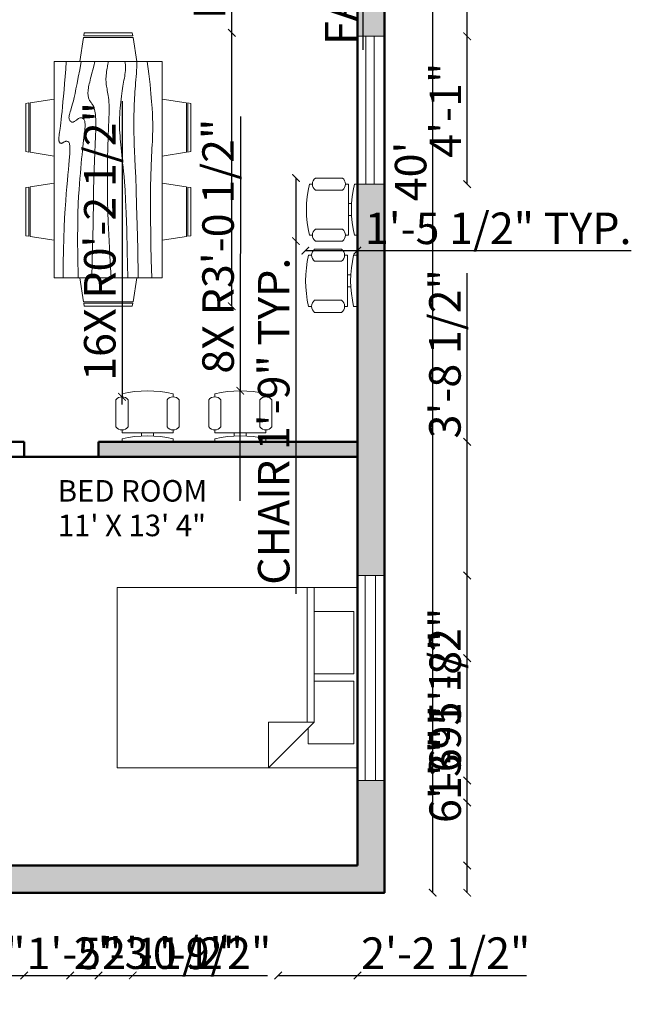
# Model space of a CAD drawing. Units: inches. Extents: x 1699 to 2290, y 1404 to 1978.
# Tile 3 of 4: x 2086 to 2290, y 1404 to 1732. Entities that reach past the tile are written whole.
import ezdxf

# ---------------------------------------------------------------- set-up
doc = ezdxf.new("R2010")
doc.units = ezdxf.units.IN
for name, color, linetype, lineweight in [('A-ANNO-DIMS', 2, 'Continuous', 18), ('A-AREA-IDEN', 7, 'Continuous', 25), ('A-FURN', 8, 'Continuous', 18), ('A-WALL', 7, 'Continuous', 50), ('A-WALL-PATT', 17, 'Continuous', 13), ('window', 3, 'Continuous', 18)]:
    doc.layers.add(name, color=color, linetype=linetype, lineweight=lineweight)
doc.styles.get("Standard").update_dxf_attribs({"font": 'arial.ttf'})
doc.dimstyles.new('ISO-25', dxfattribs={"dimtxt": 10.5, "dimasz": 2.5, "dimexe": 1.25, "dimexo": 0.625, "dimtad": 1, "dimdec": 0, "dimlunit": 4, "dimtxsty": 'Standard', "dimblk": 'ARCHTICK', "dimcen": 2.5, "dimse1": 1, "dimse2": 1, "dimclrd": 4, "dimclrt": 2, "dimadec": 0, "dimazin": 0, "dimtfac": 1, "dimtdec": 0, "dimtmove": 0, "dimatfit": 3, "dimfxl": 1, "dimarcsym": 0})

# ---------------------------------------------------------------- blocks, each defined once
blk = doc.blocks.new('Bed - Queen')
for p, q in [((0, -80.00003), (0, 0)), ((0, 0), (59.99999, 0)), ((59.99999, 0), (59.99999, -80.00003)), ((7.99999, -1.2), (28.79998, -1.2)), ((7.99999, -14.4), (7.99999, -1.2)), ((28.79998, -1.2), (28.79998, -14.4)), ((31.19999, -1.2), (51.99999, -1.2)), ((31.19999, -14.4), (31.19999, -1.2)), ((51.99999, -1.2), (51.99999, -16.4)), ((0, -14.4), (44.8, -14.4)), ((59.99999, -29.6), (44.8, -14.4)), ((44.8, -14.4), (44.8, -29.6)), ((44.8, -16.8), (0, -16.8)), ((51.99999, -16.4), (46.79936, -16.4)), ((44.8, -29.6), (59.99999, -29.6)), ((59.99999, -80.00003), (0, -80.00003))]:
    blk.add_line(p, q)
blk = doc.blocks.new('Dining Set - 36 x 72 in.')
for p, q in [((-22, 27.5), (-22.1562, 26.50042)), ((-5.8416, 26.5), (-22.1534, 26.5)), ((-22, 27.5), (-6, 27.5)), ((-5.8437, 26.49966), (-6, 27.5)), ((6, 27.5), (5.8438, 26.50042)), ((22.1584, 26.5), (5.8466, 26.5)), ((6, 27.5), (22, 27.5)), ((22.1563, 26.49966), (22, 27.5)), ((-22.2343, 26.00059), (-23.4847, 17.99762)), ((-22.2304, 26), (-5.7608, 26)), ((-4.5152, 17.99762), (-5.7655, 25.99926)), ((5.7657, 26.00059), (4.5153, 17.99762)), ((5.7696, 26), (22.2392, 26)), ((23.4848, 17.99762), (22.2345, 25.99926)), ((36, 18), (-36, 18)), ((-36, 18), (-36, -18)), ((36, -18), (36, 18)), ((-45.5, 8), (-44.5004, 8.15617)), ((-45.5, 8), (-45.5, -8)), ((-44.5, -8.15843), (-44.5, 8.15338)), ((-44.0006, 8.23428), (-35.9976, 9.48474)), ((-44, 8.23041), (-44, -8.23915)), ((44.0006, 8.23428), (35.9976, 9.48474)), ((44, 8.23041), (44, -8.23915)), ((44.5, -8.15843), (44.5, 8.15338)), ((45.5, 8), (44.5005, 8.15617)), ((45.5, 8), (45.5, -8)), ((-44.4997, -8.15631), (-45.5, -8)), ((-35.9976, -9.48476), (-43.9993, -8.2345)), ((35.9976, -9.48476), (43.9993, -8.2345)), ((44.4997, -8.15631), (45.5, -8)), ((-36, -18), (36, -18)), ((-22.2343, -26.0006), (-23.4847, -17.99762)), ((-4.5152, -17.99762), (-5.7655, -25.99928)), ((5.7657, -26.0006), (4.5153, -17.99762)), ((23.4848, -17.99762), (22.2345, -25.99928)), ((-22.2304, -26), (-5.7608, -26)), ((5.7696, -26), (22.2392, -26)), ((-22, -27.5), (-22.1562, -26.50044)), ((-5.8416, -26.5), (-22.1534, -26.5)), ((-22, -27.5), (-6, -27.5)), ((-5.8437, -26.49967), (-6, -27.5)), ((6, -27.5), (5.8438, -26.50044)), ((22.1584, -26.5), (5.8466, -26.5)), ((6, -27.5), (22, -27.5)), ((22.1563, -26.49967), (22, -27.5))]:
    blk.add_line(p, q)
for points in [[(-36, 15), (-31.1772, 14.97754), (-26.8079, 14.91406), (-22.8538, 14.81543), (-19.276, 14.6875), (-16.0362, 14.53613), (-13.0957, 14.36718), (-10.4159, 14.18652), (-7.9583, 14), (-5.6904, 13.81315), (-3.6035, 13.63021), (-1.6954, 13.45508), (0.0365, 13.29166), (1.5945, 13.14388), (2.9811, 13.01562), (4.1988, 12.9108), (5.25, 12.83333), (6.1393, 12.78613), (6.8802, 12.76823), (7.4883, 12.77767), (7.9792, 12.8125), (8.3685, 12.87077), (8.6719, 12.95052), (8.9049, 13.0498), (9.0833, 13.16666), (9.2205, 13.29899), (9.3216, 13.44401), (9.3895, 13.59879), (9.4271, 13.76041), (9.4373, 13.92594), (9.4232, 14.09245), (9.3875, 14.257), (9.3333, 14.41666), (9.2638, 14.56917), (9.1836, 14.71484), (9.0975, 14.85465), (9.0104, 14.98958), (8.9272, 15.1206), (8.8529, 15.2487), (8.7922, 15.37483), (8.75, 15.5), (8.7305, 15.62467), (8.7344, 15.74739), (8.7617, 15.86621), (8.8125, 15.97916), (8.8867, 16.08431), (8.9844, 16.17968), (9.1055, 16.26334), (9.25, 16.33333), (9.4189, 16.38802), (9.6172, 16.42708), (9.8506, 16.45052), (10.125, 16.45833), (10.4463, 16.45052), (10.8203, 16.42708), (11.2529, 16.38802), (11.75, 16.33333), (12.3184, 16.26318), (12.9694, 16.17838), (13.7151, 16.07991), (14.5677, 15.96875), (15.5395, 15.84586), (16.6426, 15.71224), (17.8893, 15.56884), (19.2917, 15.41666), (20.859, 15.25667), (22.5879, 15.08984), (24.4721, 14.91715), (26.5052, 14.73958), (28.6809, 14.5581), (30.9929, 14.3737), (33.4347, 14.18733), (36, 14)], [(-36, 10), (-28.9766, 10.14274), (-23.1725, 10.20442), (-18.4241, 10.19775), (-14.5677, 10.13541), (-11.4399, 10.03011), (-8.877, 9.89453), (-6.7154, 9.74137), (-4.7917, 9.58333), (-2.9698, 9.43082), (-1.2246, 9.28515), (0.4415, 9.14534), (2.026, 9.01041), (3.5266, 8.87939), (4.9408, 8.7513), (6.266, 8.62516), (7.5, 8.5), (8.6411, 8.37549), (9.6914, 8.2539), (10.6538, 8.13818), (11.5312, 8.03125), (12.3267, 7.93603), (13.043, 7.85547), (13.6831, 7.79248), (14.25, 7.75), (14.7471, 7.7303), (15.1797, 7.73307), (15.5537, 7.75732), (15.875, 7.80208), (16.1494, 7.86637), (16.3828, 7.94922), (16.5811, 8.04964), (16.75, 8.16666), (16.8944, 8.29915), (17.0143, 8.44531), (17.1089, 8.60319), (17.1771, 8.77083), (17.218, 8.94629), (17.2305, 9.1276), (17.2137, 9.31282), (17.1667, 9.5), (17.0895, 9.6875), (16.987, 9.875), (16.8649, 10.0625), (16.7292, 10.25), (16.5856, 10.4375), (16.4401, 10.625), (16.2985, 10.8125), (16.1667, 11), (16.05, 11.18733), (15.9518, 11.3737), (15.8752, 11.5581), (15.8229, 11.73958), (15.798, 11.91715), (15.8034, 12.08984), (15.842, 12.25667), (15.9167, 12.41666), (16.0295, 12.56836), (16.1784, 12.70833), (16.3605, 12.83268), (16.5729, 12.9375), (16.8127, 13.01888), (17.0768, 13.07291), (17.3625, 13.0957), (17.6667, 13.08333), (17.9894, 13.03312), (18.3418, 12.94726), (18.7382, 12.82918), (19.1927, 12.68229), (19.7195, 12.51001), (20.3327, 12.31575), (21.0465, 12.10294), (21.875, 11.875), (22.8357, 11.63354), (23.959, 11.37304), (25.2786, 11.08618), (26.8282, 10.76562), (28.6414, 10.40405), (30.752, 9.99414), (33.1936, 9.52856), (36, 9)], [(-36, 5.5), (-30.7157, 5.3348), (-26.069, 5.20963), (-21.9946, 5.11767), (-18.4271, 5.05208), (-15.3009, 5.00602), (-12.5508, 4.97265), (-10.1112, 4.94515), (-7.9167, 4.91666), (-5.909, 4.88167), (-4.0586, 4.83984), (-2.3429, 4.79215), (-0.7396, 4.73958), (0.7739, 4.6831), (2.22, 4.6237), (3.6213, 4.56233), (5, 4.5), (6.373, 4.43782), (7.7344, 4.3776), (9.0723, 4.32129), (10.375, 4.27083), (11.6309, 4.22819), (12.8281, 4.19531), (13.9551, 4.17415), (15, 4.16666), (15.954, 4.17448), (16.819, 4.19791), (17.6001, 4.23698), (18.3021, 4.29166), (18.9299, 4.36198), (19.4883, 4.44791), (19.9823, 4.54948), (20.4167, 4.66666), (20.7969, 4.79899), (21.1302, 4.94401), (21.4245, 5.09879), (21.6875, 5.26041), (21.9271, 5.42594), (22.1511, 5.59245), (22.3672, 5.757), (22.5834, 5.91666), (22.8065, 6.06868), (23.0404, 6.21093), (23.2879, 6.34147), (23.5521, 6.45833), (23.8358, 6.55957), (24.142, 6.64323), (24.4735, 6.70735), (24.8334, 6.75), (25.2235, 6.76969), (25.642, 6.76692), (26.0858, 6.74267), (26.5521, 6.69791), (27.0379, 6.63362), (27.5404, 6.55078), (28.0565, 6.45036), (28.5834, 6.33333), (29.1242, 6.19987), (29.7071, 6.04687), (30.3661, 5.87044), (31.1354, 5.66666), (32.0493, 5.43164), (33.142, 5.16146), (34.4475, 4.85221), (36, 4.5)], [(-36, -1), (-30.7915, -0.6591), (-26.0195, -0.38216), (-21.6519, -0.16284), (-17.6563, 0.00521), (-14.0005, 0.12833), (-10.6523, 0.21289), (-7.5796, 0.26522), (-4.75, 0.29166), (-2.134, 0.29793), (0.2878, 0.28711), (2.5317, 0.26163), (4.6146, 0.22396), (6.5529, 0.17651), (8.3633, 0.12174), (10.0623, 0.06209), (11.6667, 0), (13.1899, -0.06201), (14.6341, -0.1211), (15.9982, -0.17432), (17.2813, -0.21875), (18.4823, -0.25147), (19.6003, -0.26953), (20.6343, -0.27002), (21.5834, -0.25), (22.4481, -0.20768), (23.2357, -0.14584), (23.9549, -0.06836), (24.6146, 0.02083), (25.2235, 0.11784), (25.7904, 0.21875), (26.3241, 0.31966), (26.8334, 0.41666), (27.3265, 0.50618), (27.8099, 0.58593), (28.2894, 0.65397), (28.7709, 0.70833), (29.2601, 0.74707), (29.763, 0.76823), (30.2855, 0.76985), (30.8334, 0.75), (31.4088, 0.70784), (31.9994, 0.64713), (32.589, 0.57275), (33.1615, 0.48958), (33.7008, 0.4025), (34.1908, 0.3164), (34.6153, 0.23616), (34.9584, 0.16666), (35.2099, 0.11165), (35.3848, 0.07031), (35.504, 0.04069), (35.5886, 0.02083), (35.6594, 0.00879), (35.7377, 0.0026), (35.8442, 0.00032), (36, 0)], [(-36, -6.5), (-27.1843, -6.31267), (-20.084, -6.1263), (-14.469, -5.9419), (-10.1094, -5.76042), (-6.7752, -5.58285), (-4.2363, -5.41016), (-2.2629, -5.24333), (-0.625, -5.08334), (0.8708, -4.93099), (2.2715, -4.78646), (3.5872, -4.64974), (4.8281, -4.52084), (6.0046, -4.39974), (7.127, -4.28646), (8.2053, -4.18099), (9.25, -4.08334), (10.2705, -3.99382), (11.2734, -3.91407), (12.2647, -3.84603), (13.25, -3.79167), (14.2354, -3.75293), (15.2266, -3.73177), (16.2295, -3.73015), (17.25, -3.75), (18.2912, -3.79248), (19.3451, -3.85547), (20.4009, -3.93604), (21.4479, -4.03125), (22.4754, -4.13819), (23.4727, -4.25391), (24.4289, -4.37549), (25.3334, -4.5), (26.1785, -4.62492), (26.9694, -4.74935), (27.7145, -4.87281), (28.4219, -4.99479), (29.1, -5.11483), (29.7572, -5.23242), (30.4016, -5.34709), (31.0417, -5.45834), (31.6837, -5.56437), (32.3262, -5.65821), (32.9658, -5.73153), (33.599, -5.77604), (34.2224, -5.78345), (34.8327, -5.74545), (35.4264, -5.65373), (36, -5.5)], [(-36, -10), (-26.4022, -9.81299), (-18.4675, -9.62891), (-11.9839, -9.45069), (-6.7396, -9.28125), (-2.5226, -9.12354), (0.8789, -8.98047), (3.6769, -8.85498), (6.0833, -8.75), (8.2767, -8.66765), (10.3021, -8.60677), (12.1712, -8.56543), (13.8958, -8.54167), (15.4876, -8.53353), (16.9583, -8.53907), (18.3197, -8.55632), (19.5834, -8.58334), (20.7616, -8.61841), (21.8685, -8.66081), (22.9188, -8.71004), (23.9271, -8.76563), (24.9081, -8.82707), (25.8763, -8.89388), (26.8465, -8.96558), (27.8334, -9.04167), (28.8474, -9.12118), (29.8828, -9.20117), (30.93, -9.27824), (31.9792, -9.34896), (33.0205, -9.40991), (34.0443, -9.45768), (35.0407, -9.48885), (36, -9.5)], [(-36, -14.5), (-30.0881, -14.33513), (-25.0332, -14.21224), (-20.7312, -14.12647), (-17.0781, -14.07292), (-13.97, -14.04671), (-11.3027, -14.04297), (-8.9724, -14.05681), (-6.875, -14.08334), (-4.9224, -14.11833), (-3.0905, -14.16016), (-1.3709, -14.20785), (0.2448, -14.26042), (1.7647, -14.3169), (3.1973, -14.3763), (4.5507, -14.43767), (5.8333, -14.5), (7.0554, -14.5621), (8.235, -14.62175), (9.3922, -14.67652), (10.5469, -14.72396), (11.7192, -14.76164), (12.929, -14.78711), (14.1965, -14.79794), (15.5417, -14.79167), (16.9933, -14.76424), (18.6152, -14.70508), (20.4804, -14.60197), (22.6615, -14.44271), (25.2312, -14.21509), (28.2624, -13.9069), (31.8277, -13.50594), (36, -13)]]:
    blk.add_lwpolyline(points)
blk = doc.blocks.new('Chair - Desk')
for p, q in [((-8.5, 0), (-8.5, -1)), ((-8.5, 0), (8.5, 0)), ((8.5, 0), (8.5, -1)), ((-8.5, -3), (-8.5, -4)), ((-8.5, -3), (8.5, -3)), ((-2, -3), (-2, -1.9355)), ((2, -1.9576), (2, -3)), ((8.5, -3), (8.5, -4)), ((-10.5, -5), (-10.5, -14)), ((-6.5, -14), (-6.5, -5)), ((6.5, -5), (6.5, -14)), ((10.5, -14), (10.5, -5)), ((-8.5, -15), (-8.5, -16)), ((8.5, -15), (8.5, -16))]:
    blk.add_line(p, q)
for centre, radius, start, end in [((0, 34.625), 36.625, 256.5803, 283.4197), ((-8.5, -6.5), 2.5, 36.8699, 143.1301), ((8.5, -6.5), 2.5, 36.8699, 143.1301), ((-8.5, -12.5), 2.5, 216.8699, 323.1301), ((0, 19.625), 36.625, 256.5803, 283.4197), ((8.5, -12.5), 2.5, 216.8699, 323.1301)]:
    blk.add_arc(centre, radius, start, end)
blk = doc.blocks.new('_ArchTick')
at = {"color": 0, "linetype": 'ByBlock', "const_width": 0.15}
blk.add_lwpolyline([(-0.5, -0.5), (0.5, 0.5)], dxfattribs=at)
blk = doc.blocks.new('*D11')
at = {"layer": 'A-ANNO-DIMS', "color": 0, "lineweight": -2, "transparency": 16777216}
blk.add_line((2223.88, 1441.58), (2223.88, 1921.58), dxfattribs=at)
at = {"layer": 'Defpoints', "color": 0, "transparency": 16777216}
for p in [(2207.82, 1921.58), (2223.88, 1921.58), (2207.82, 1441.58)]:
    blk.add_point(p, dxfattribs=at)
at = {"layer": 'A-ANNO-DIMS', "color": 0, "lineweight": -2, "transparency": 16777216, "xscale": 2.5, "yscale": 2.5, "zscale": 2.5}
for p, rotation in [((2223.88, 1921.58), 90), ((2223.88, 1441.58), 270)]:
    blk.add_blockref('_ArchTick', p, dxfattribs=dict(at, rotation=rotation))
at = {"layer": 'A-ANNO-DIMS', "color": 0, "transparency": 16777216, "insert": (2217.89, 1681.58), "char_height": 10.5, "attachment_point": 5, "rotation": 90}
blk.add_mtext("40'", dxfattribs=at)
blk = doc.blocks.new('*D14')
at = {"layer": 'A-ANNO-DIMS', "color": 4, "lineweight": -2, "transparency": 16777216}
for p, q in [((2178.34, 1679.38), (2178.34, 1658.38)), ((2178.34, 1658.38), (2178.34, 1541.04))]:
    blk.add_line(p, q, dxfattribs=at)
at = {"layer": 'Defpoints', "color": 0, "transparency": 16777216}
for p in [(2181.49, 1679.38), (2178.34, 1658.38), (2181.49, 1658.38)]:
    blk.add_point(p, dxfattribs=at)
at = {"layer": 'A-ANNO-DIMS', "color": 4, "lineweight": -2, "transparency": 16777216, "xscale": 2.5, "yscale": 2.5, "zscale": 2.5}
for p, rotation in [((2178.34, 1679.38), 90), ((2178.34, 1658.38), 270)]:
    blk.add_blockref('_ArchTick', p, dxfattribs=dict(at, rotation=rotation))
at = {"layer": 'A-ANNO-DIMS', "color": 2, "transparency": 16777216, "insert": (2172.28, 1598.46), "char_height": 10.5, "attachment_point": 5, "rotation": 90}
blk.add_mtext('CHAIR 1\'-9" TYP.', dxfattribs=at)
blk = doc.blocks.new('*D15')
at = {"layer": 'A-ANNO-DIMS', "color": 4, "lineweight": -2, "transparency": 16777216}
for p, q in [((2181.49, 1655.23), (2198.82, 1655.23)), ((2198.82, 1655.23), (2290.05, 1655.23))]:
    blk.add_line(p, q, dxfattribs=at)
at = {"layer": 'Defpoints', "color": 0, "transparency": 16777216}
for p in [(2181.49, 1658.38), (2198.82, 1658.38), (2198.82, 1655.23)]:
    blk.add_point(p, dxfattribs=at)
at = {"layer": 'A-ANNO-DIMS', "color": 4, "lineweight": -2, "transparency": 16777216, "xscale": 2.5, "yscale": 2.5, "zscale": 2.5, "rotation": 180}
blk.add_blockref('_ArchTick', (2181.49, 1655.23), dxfattribs=at)
at = {"layer": 'A-ANNO-DIMS', "color": 4, "lineweight": -2, "transparency": 16777216, "xscale": 2.5, "yscale": 2.5, "zscale": 2.5}
blk.add_blockref('_ArchTick', (2198.82, 1655.23), dxfattribs=at)
at = {"layer": 'A-ANNO-DIMS', "color": 2, "transparency": 16777216, "insert": (2245.69, 1661.29), "char_height": 10.5, "attachment_point": 5}
blk.add_mtext('1\'-5 1/2" TYP.', dxfattribs=at)
blk = doc.blocks.new('*D16')
at = {"layer": 'A-ANNO-DIMS', "color": 4, "lineweight": -2, "transparency": 16777216}
for p, q in [((2156.97, 1727.7), (2156.97, 1846.86)), ((2156.97, 1636.7), (2156.97, 1727.7))]:
    blk.add_line(p, q, dxfattribs=at)
at = {"layer": 'Defpoints', "color": 0, "transparency": 16777216}
for p in [(2143.32, 1727.7), (2156.97, 1727.7), (2143.32, 1636.7)]:
    blk.add_point(p, dxfattribs=at)
at = {"layer": 'A-ANNO-DIMS', "color": 4, "lineweight": -2, "transparency": 16777216, "xscale": 2.5, "yscale": 2.5, "zscale": 2.5}
for p, rotation in [((2156.97, 1727.7), 90), ((2156.97, 1636.7), 270)]:
    blk.add_blockref('_ArchTick', p, dxfattribs=dict(at, rotation=rotation))
at = {"layer": 'A-ANNO-DIMS', "color": 2, "transparency": 16777216, "insert": (2150.92, 1788.53), "char_height": 10.5, "attachment_point": 5, "rotation": 90}
blk.add_mtext('DINING SET 7\'-7"', dxfattribs=at)
blk = doc.blocks.new('*D17')
at = {"layer": 'A-ANNO-DIMS', "color": 4, "lineweight": -2, "transparency": 16777216}
blk.add_line((2143.32, 1741.35), (2088.32, 1741.35), dxfattribs=at)
at = {"layer": 'Defpoints', "color": 0, "transparency": 16777216}
for p in [(2088.32, 1741.35), (2088.32, 1727.7), (2143.32, 1727.7)]:
    blk.add_point(p, dxfattribs=at)
at = {"layer": 'A-ANNO-DIMS', "color": 4, "lineweight": -2, "transparency": 16777216, "xscale": 2.5, "yscale": 2.5, "zscale": 2.5, "rotation": 180}
blk.add_blockref('_ArchTick', (2088.32, 1741.35), dxfattribs=at)
at = {"layer": 'A-ANNO-DIMS', "color": 4, "lineweight": -2, "transparency": 16777216, "xscale": 2.5, "yscale": 2.5, "zscale": 2.5}
blk.add_blockref('_ArchTick', (2143.32, 1741.35), dxfattribs=at)
at = {"layer": 'A-ANNO-DIMS', "color": 2, "transparency": 16777216, "insert": (2115.82, 1747.22), "char_height": 10.5, "attachment_point": 5}
blk.add_mtext('4\'-7"', dxfattribs=at)
blk = doc.blocks.new('*D22')
at = {"layer": 'A-ANNO-DIMS', "color": 4, "lineweight": -2, "transparency": 16777216}
for p, q in [((2200.62, 1827.84), (2200.62, 1815.84)), ((2200.62, 1815.84), (2200.62, 1722.02))]:
    blk.add_line(p, q, dxfattribs=at)
at = {"layer": 'Defpoints', "color": 0, "transparency": 16777216}
for p in [(2198.82, 1827.84), (2198.82, 1815.84), (2200.62, 1815.84)]:
    blk.add_point(p, dxfattribs=at)
at = {"layer": 'A-ANNO-DIMS', "color": 4, "lineweight": -2, "transparency": 16777216, "xscale": 2.5, "yscale": 2.5, "zscale": 2.5}
for p, rotation in [((2200.62, 1827.84), 90), ((2200.62, 1815.84), 270)]:
    blk.add_blockref('_ArchTick', p, dxfattribs=dict(at, rotation=rotation))
at = {"layer": 'A-ANNO-DIMS', "color": 2, "transparency": 16777216, "insert": (2194.57, 1767.68), "char_height": 10.5, "attachment_point": 5, "rotation": 90}
blk.add_mtext('FAUCET 1\'-0"', dxfattribs=at)
blk = doc.blocks.new('*D36')
at = {"layer": 'A-ANNO-DIMS', "color": 4, "lineweight": -2, "transparency": 16777216}
for p, q in [((2235.37, 1478.94), (2235.37, 1535.06)), ((2235.37, 1441.58), (2235.37, 1478.94))]:
    blk.add_line(p, q, dxfattribs=at)
at = {"layer": 'Defpoints', "color": 0, "transparency": 16777216}
for p in [(2207.82, 1478.94), (2235.37, 1478.94), (2207.82, 1441.58)]:
    blk.add_point(p, dxfattribs=at)
at = {"layer": 'A-ANNO-DIMS', "color": 4, "lineweight": -2, "transparency": 16777216, "xscale": 2.5, "yscale": 2.5, "zscale": 2.5}
for p, rotation in [((2235.37, 1478.94), 90), ((2235.37, 1441.58), 270)]:
    blk.add_blockref('_ArchTick', p, dxfattribs=dict(at, rotation=rotation))
at = {"layer": 'A-ANNO-DIMS', "color": 2, "transparency": 16777216, "insert": (2229.31, 1508.25), "char_height": 10.5, "attachment_point": 5, "rotation": 90}
blk.add_mtext('3\'-1 1/2"', dxfattribs=at)
blk = doc.blocks.new('*D37')
at = {"layer": 'A-ANNO-DIMS', "color": 4, "lineweight": -2, "transparency": 16777216}
blk.add_line((2235.37, 1478.94), (2235.37, 1547.09), dxfattribs=at)
at = {"layer": 'Defpoints', "color": 0, "transparency": 16777216}
for p in [(2207.82, 1547.09), (2235.37, 1547.09), (2207.82, 1478.94)]:
    blk.add_point(p, dxfattribs=at)
at = {"layer": 'A-ANNO-DIMS', "color": 4, "lineweight": -2, "transparency": 16777216, "xscale": 2.5, "yscale": 2.5, "zscale": 2.5}
for p, rotation in [((2235.37, 1547.09), 90), ((2235.37, 1478.94), 270)]:
    blk.add_blockref('_ArchTick', p, dxfattribs=dict(at, rotation=rotation))
at = {"layer": 'A-ANNO-DIMS', "color": 2, "transparency": 16777216, "insert": (2229.39, 1513.01), "char_height": 10.5, "attachment_point": 5, "rotation": 90}
blk.add_mtext('5\'-8"', dxfattribs=at)
blk = doc.blocks.new('*D38')
at = {"layer": 'A-ANNO-DIMS', "color": 4, "lineweight": -2, "transparency": 16777216}
for p, q in [((2235.37, 1591.58), (2235.37, 1647.71)), ((2235.37, 1547.09), (2235.37, 1591.58))]:
    blk.add_line(p, q, dxfattribs=at)
at = {"layer": 'Defpoints', "color": 0, "transparency": 16777216}
for p in [(2198.82, 1591.58), (2235.37, 1591.58), (2207.82, 1547.09)]:
    blk.add_point(p, dxfattribs=at)
at = {"layer": 'A-ANNO-DIMS', "color": 4, "lineweight": -2, "transparency": 16777216, "xscale": 2.5, "yscale": 2.5, "zscale": 2.5}
for p, rotation in [((2235.37, 1591.58), 90), ((2235.37, 1547.09), 270)]:
    blk.add_blockref('_ArchTick', p, dxfattribs=dict(at, rotation=rotation))
at = {"layer": 'A-ANNO-DIMS', "color": 2, "transparency": 16777216, "insert": (2229.31, 1620.9), "char_height": 10.5, "attachment_point": 5, "rotation": 90}
blk.add_mtext('3\'-8 1/2"', dxfattribs=at)
blk = doc.blocks.new('*D39')
at = {"layer": 'A-ANNO-DIMS', "color": 4, "lineweight": -2, "transparency": 16777216}
blk.add_line((2235.37, 1677.38), (2235.37, 1726.54), dxfattribs=at)
at = {"layer": 'Defpoints', "color": 0, "transparency": 16777216}
for p in [(2207.82, 1726.54), (2235.37, 1726.54), (2207.82, 1677.38)]:
    blk.add_point(p, dxfattribs=at)
at = {"layer": 'A-ANNO-DIMS', "color": 4, "lineweight": -2, "transparency": 16777216, "xscale": 2.5, "yscale": 2.5, "zscale": 2.5}
for p, rotation in [((2235.37, 1726.54), 90), ((2235.37, 1677.38), 270)]:
    blk.add_blockref('_ArchTick', p, dxfattribs=dict(at, rotation=rotation))
at = {"layer": 'A-ANNO-DIMS', "color": 2, "transparency": 16777216, "insert": (2229.48, 1701.96), "char_height": 10.5, "attachment_point": 5, "rotation": 90}
blk.add_mtext('4\'-1"', dxfattribs=at)
blk = doc.blocks.new('*D40')
at = {"layer": 'A-ANNO-DIMS', "color": 4, "lineweight": -2, "transparency": 16777216}
blk.add_line((2235.37, 1726.54), (2235.37, 1780.58), dxfattribs=at)
at = {"layer": 'Defpoints', "color": 0, "transparency": 16777216}
for p in [(2198.82, 1780.58), (2235.37, 1780.58), (2207.82, 1726.54)]:
    blk.add_point(p, dxfattribs=at)
at = {"layer": 'A-ANNO-DIMS', "color": 4, "lineweight": -2, "transparency": 16777216, "xscale": 2.5, "yscale": 2.5, "zscale": 2.5}
for p, rotation in [((2235.37, 1780.58), 90), ((2235.37, 1726.54), 270)]:
    blk.add_blockref('_ArchTick', p, dxfattribs=dict(at, rotation=rotation))
at = {"layer": 'A-ANNO-DIMS', "color": 2, "transparency": 16777216, "insert": (2229.39, 1753.56), "char_height": 10.5, "attachment_point": 5, "rotation": 90}
blk.add_mtext('4\'-6"', dxfattribs=at)
blk = doc.blocks.new('*D42')
at = {"layer": 'A-ANNO-DIMS', "color": 4, "lineweight": -2, "transparency": 16777216}
for p, q in [((2172.42, 1414.03), (2198.82, 1414.03)), ((2198.82, 1414.03), (2255.13, 1414.03))]:
    blk.add_line(p, q, dxfattribs=at)
at = {"layer": 'Defpoints', "color": 0, "transparency": 16777216}
for p in [(2172.42, 1785.58), (2198.82, 1785.58), (2198.82, 1414.03)]:
    blk.add_point(p, dxfattribs=at)
at = {"layer": 'A-ANNO-DIMS', "color": 4, "lineweight": -2, "transparency": 16777216, "xscale": 2.5, "yscale": 2.5, "zscale": 2.5, "rotation": 180}
blk.add_blockref('_ArchTick', (2172.42, 1414.03), dxfattribs=at)
at = {"layer": 'A-ANNO-DIMS', "color": 4, "lineweight": -2, "transparency": 16777216, "xscale": 2.5, "yscale": 2.5, "zscale": 2.5}
blk.add_blockref('_ArchTick', (2198.82, 1414.03), dxfattribs=at)
at = {"layer": 'A-ANNO-DIMS', "color": 2, "transparency": 16777216, "insert": (2228.23, 1420.09), "char_height": 10.5, "attachment_point": 5}
blk.add_mtext('2\'-2 1/2"', dxfattribs=at)
blk = doc.blocks.new('*D53')
at = {"layer": 'A-ANNO-DIMS', "color": 4, "lineweight": -2, "transparency": 16777216}
for p, q in [((2087.8, 1414.03), (2112.54, 1414.03)), ((2112.54, 1414.03), (2168.85, 1414.03))]:
    blk.add_line(p, q, dxfattribs=at)
at = {"layer": 'Defpoints', "color": 0, "transparency": 16777216}
for p in [(2087.8, 1586.58), (2112.54, 1586.58), (2112.54, 1414.03)]:
    blk.add_point(p, dxfattribs=at)
at = {"layer": 'A-ANNO-DIMS', "color": 4, "lineweight": -2, "transparency": 16777216, "xscale": 2.5, "yscale": 2.5, "zscale": 2.5, "rotation": 180}
blk.add_blockref('_ArchTick', (2087.8, 1414.03), dxfattribs=at)
at = {"layer": 'A-ANNO-DIMS', "color": 4, "lineweight": -2, "transparency": 16777216, "xscale": 2.5, "yscale": 2.5, "zscale": 2.5}
blk.add_blockref('_ArchTick', (2112.54, 1414.03), dxfattribs=at)
at = {"layer": 'A-ANNO-DIMS', "color": 2, "transparency": 16777216, "insert": (2141.95, 1420.09), "char_height": 10.5, "attachment_point": 5}
blk.add_mtext('2\'-0 1/2"', dxfattribs=at)
blk = doc.blocks.new('*D58')
at = {"layer": 'A-ANNO-DIMS', "color": 4, "lineweight": -2, "transparency": 16777216}
for p, q in [((2235.37, 1471.58), (2235.37, 1502.26)), ((2235.37, 1450.58), (2235.37, 1471.58))]:
    blk.add_line(p, q, dxfattribs=at)
at = {"layer": 'Defpoints', "color": 0, "transparency": 16777216}
for p in [(1864.82, 1471.58), (2235.37, 1471.58), (1864.82, 1450.58)]:
    blk.add_point(p, dxfattribs=at)
at = {"layer": 'A-ANNO-DIMS', "color": 4, "lineweight": -2, "transparency": 16777216, "xscale": 2.5, "yscale": 2.5, "zscale": 2.5}
for p, rotation in [((2235.37, 1471.58), 90), ((2235.37, 1450.58), 270)]:
    blk.add_blockref('_ArchTick', p, dxfattribs=dict(at, rotation=rotation))
at = {"layer": 'A-ANNO-DIMS', "color": 2, "transparency": 16777216, "insert": (2229.39, 1488.17), "char_height": 10.5, "attachment_point": 5, "rotation": 90}
blk.add_mtext('1\'-9"', dxfattribs=at)
blk = doc.blocks.new('*D60')
at = {"layer": 'A-ANNO-DIMS', "color": 4, "lineweight": -2, "transparency": 16777216}
blk.add_line((2235.37, 1441.58), (2235.37, 1519.58), dxfattribs=at)
at = {"layer": 'Defpoints', "color": 0, "transparency": 16777216}
for p in [(2005.82, 1519.58), (2235.37, 1519.58), (1847.82, 1441.58)]:
    blk.add_point(p, dxfattribs=at)
at = {"layer": 'A-ANNO-DIMS', "color": 4, "lineweight": -2, "transparency": 16777216, "xscale": 2.5, "yscale": 2.5, "zscale": 2.5}
for p, rotation in [((2235.37, 1519.58), 90), ((2235.37, 1441.58), 270)]:
    blk.add_blockref('_ArchTick', p, dxfattribs=dict(at, rotation=rotation))
at = {"layer": 'A-ANNO-DIMS', "color": 2, "transparency": 16777216, "insert": (2229.39, 1480.58), "char_height": 10.5, "attachment_point": 5, "rotation": 90}
blk.add_mtext('6\'-6"', dxfattribs=at)
blk = doc.blocks.new('*D61')
at = {"layer": 'A-ANNO-DIMS', "color": 4, "lineweight": -2, "transparency": 16777216}
for p, q in [((2000.82, 1414.03), (2023.18, 1414.03)), ((2023.18, 1414.03), (2086.48, 1414.03))]:
    blk.add_line(p, q, dxfattribs=at)
at = {"layer": 'Defpoints', "color": 0, "transparency": 16777216}
for p in [(2000.82, 1842.58), (2023.18, 1842.58), (2023.18, 1414.03)]:
    blk.add_point(p, dxfattribs=at)
at = {"layer": 'A-ANNO-DIMS', "color": 4, "lineweight": -2, "transparency": 16777216, "xscale": 2.5, "yscale": 2.5, "zscale": 2.5, "rotation": 180}
blk.add_blockref('_ArchTick', (2000.82, 1414.03), dxfattribs=at)
at = {"layer": 'A-ANNO-DIMS', "color": 4, "lineweight": -2, "transparency": 16777216, "xscale": 2.5, "yscale": 2.5, "zscale": 2.5}
blk.add_blockref('_ArchTick', (2023.18, 1414.03), dxfattribs=at)
at = {"layer": 'A-ANNO-DIMS', "color": 2, "transparency": 16777216, "insert": (2056.08, 1420.09), "char_height": 10.5, "attachment_point": 5}
blk.add_mtext('1\'-10 1/2"', dxfattribs=at)
blk = doc.blocks.new('*D62')
at = {"layer": 'A-ANNO-DIMS', "color": 4, "lineweight": -2, "transparency": 16777216}
for p, q in [((2070.82, 1414.03), (2087.8, 1414.03)), ((2087.8, 1414.03), (2118.47, 1414.03))]:
    blk.add_line(p, q, dxfattribs=at)
at = {"layer": 'Defpoints', "color": 0, "transparency": 16777216}
for p in [(2070.82, 1586.58), (2087.8, 1586.58), (2087.8, 1414.03)]:
    blk.add_point(p, dxfattribs=at)
at = {"layer": 'A-ANNO-DIMS', "color": 4, "lineweight": -2, "transparency": 16777216, "xscale": 2.5, "yscale": 2.5, "zscale": 2.5, "rotation": 180}
blk.add_blockref('_ArchTick', (2070.82, 1414.03), dxfattribs=at)
at = {"layer": 'A-ANNO-DIMS', "color": 4, "lineweight": -2, "transparency": 16777216, "xscale": 2.5, "yscale": 2.5, "zscale": 2.5}
blk.add_blockref('_ArchTick', (2087.8, 1414.03), dxfattribs=at)
at = {"layer": 'A-ANNO-DIMS', "color": 2, "transparency": 16777216, "insert": (2104.39, 1420.02), "char_height": 10.5, "attachment_point": 5}
blk.add_mtext('1\'-5"', dxfattribs=at)
blk = doc.blocks.new('*D67')
at = {"layer": 'A-ANNO-DIMS', "color": 4, "lineweight": -2, "transparency": 16777216}
for p, q in [((2075.82, 1414.03), (2103.12, 1414.03)), ((2103.12, 1414.03), (2159.43, 1414.03))]:
    blk.add_line(p, q, dxfattribs=at)
at = {"layer": 'Defpoints', "color": 0, "transparency": 16777216}
for p in [(2075.82, 1912.58), (2103.12, 1883.78), (2103.12, 1414.03)]:
    blk.add_point(p, dxfattribs=at)
at = {"layer": 'A-ANNO-DIMS', "color": 4, "lineweight": -2, "transparency": 16777216, "xscale": 2.5, "yscale": 2.5, "zscale": 2.5, "rotation": 180}
blk.add_blockref('_ArchTick', (2075.82, 1414.03), dxfattribs=at)
at = {"layer": 'A-ANNO-DIMS', "color": 4, "lineweight": -2, "transparency": 16777216, "xscale": 2.5, "yscale": 2.5, "zscale": 2.5}
blk.add_blockref('_ArchTick', (2103.12, 1414.03), dxfattribs=at)
at = {"layer": 'A-ANNO-DIMS', "color": 2, "transparency": 16777216, "insert": (2132.53, 1420.09), "char_height": 10.5, "attachment_point": 5}
blk.add_mtext('2\'-3 1/2"', dxfattribs=at)
blk = doc.blocks.new('*D68')
at = {"layer": 'A-ANNO-DIMS', "color": 4, "lineweight": -2, "transparency": 16777216}
for p, q in [((2103.12, 1414.03), (2123.96, 1414.03)), ((2123.96, 1414.03), (2154.63, 1414.03))]:
    blk.add_line(p, q, dxfattribs=at)
at = {"layer": 'Defpoints', "color": 0, "transparency": 16777216}
for p in [(2103.12, 1912.58), (2123.96, 1912.58), (2123.96, 1414.03)]:
    blk.add_point(p, dxfattribs=at)
at = {"layer": 'A-ANNO-DIMS', "color": 4, "lineweight": -2, "transparency": 16777216, "xscale": 2.5, "yscale": 2.5, "zscale": 2.5, "rotation": 180}
blk.add_blockref('_ArchTick', (2103.12, 1414.03), dxfattribs=at)
at = {"layer": 'A-ANNO-DIMS', "color": 4, "lineweight": -2, "transparency": 16777216, "xscale": 2.5, "yscale": 2.5, "zscale": 2.5}
blk.add_blockref('_ArchTick', (2123.96, 1414.03), dxfattribs=at)
at = {"layer": 'A-ANNO-DIMS', "color": 2, "transparency": 16777216, "insert": (2140.54, 1420.02), "char_height": 10.5, "attachment_point": 5}
blk.add_mtext('1\'-9"', dxfattribs=at)
blk = doc.blocks.new('*D73')
at = {"layer": 'A-ANNO-DIMS', "color": 4, "lineweight": -2, "transparency": 16777216}
for p in [(2159.81, 1699.84), (2159.8, 1571.96)]:
    blk.add_line(p, (2159.8, 1608.58), dxfattribs=at)
at = {"layer": 'Defpoints', "color": 0, "transparency": 16777216}
for p in [(2159.8, 1608.58), (2159.8, 1571.96)]:
    blk.add_point(p, dxfattribs=at)
at = {"layer": 'A-ANNO-DIMS', "color": 4, "lineweight": -2, "transparency": 16777216, "xscale": 2.5, "yscale": 2.5, "zscale": 2.5, "rotation": 269.9995009596273}
blk.add_blockref('_ArchTick', (2159.8, 1608.58), dxfattribs=at)
at = {"layer": 'A-ANNO-DIMS', "color": 2, "transparency": 16777216, "insert": (2153.75, 1656.71), "char_height": 10.5, "attachment_point": 5, "rotation": 89.9995}
blk.add_mtext('8X R3\'-0 1/2"', dxfattribs=at)
blk = doc.blocks.new('*D74')
at = {"layer": 'A-ANNO-DIMS', "color": 4, "lineweight": -2, "transparency": 16777216}
for p in [(2120.41, 1704.99), (2120.39, 1604.08)]:
    blk.add_line(p, (2120.39, 1606.58), dxfattribs=at)
at = {"layer": 'Defpoints', "color": 0, "transparency": 16777216}
for p in [(2120.39, 1606.58), (2120.39, 1604.08)]:
    blk.add_point(p, dxfattribs=at)
at = {"layer": 'A-ANNO-DIMS', "color": 4, "lineweight": -2, "transparency": 16777216, "xscale": 2.5, "yscale": 2.5, "zscale": 2.5, "rotation": 269.9927119768879}
blk.add_blockref('_ArchTick', (2120.39, 1606.58), dxfattribs=at)
at = {"layer": 'A-ANNO-DIMS', "color": 2, "transparency": 16777216, "insert": (2114.35, 1658.29), "char_height": 10.5, "attachment_point": 5, "rotation": 89.9927}
blk.add_mtext('16X R0\'-2 1/2"', dxfattribs=at)

msp = doc.modelspace()

# ---------------------------------------------------------------- hatches: boundary and pattern name
at = {"layer": 'A-WALL-PATT'}
h = msp.add_hatch(color=256, dxfattribs=at)
h.dxf.hatch_style = 1
h.paths.add_polyline_path([(1893.7, 1921.58), (1847.82, 1921.58), (1847.82, 1852.66), (1856.82, 1852.66), (1856.82, 1912.58), (1893.7, 1912.58)])
h.paths.add_polyline_path([(2097.62, 1921.58), (1942.38, 1921.58), (1942.38, 1912.58), (2097.62, 1912.58)])
h.paths.add_polyline_path([(2207.82, 1921.58), (2149.1, 1921.58), (2149.1, 1912.58), (2153.96, 1912.58), (2198.82, 1912.58), (2198.82, 1877.29), (2207.82, 1877.29)])
h.paths.add_polyline_path([(2207.82, 1827.84), (2198.82, 1827.84), (2198.82, 1815.84), (2198.82, 1807.65), (2198.82, 1726.54), (2207.82, 1726.54)])
h.paths.add_polyline_path([(2207.82, 1677.38), (2198.82, 1677.38), (2198.82, 1660.38), (2198.82, 1547.09), (2207.82, 1547.09)])
h.paths.add_polyline_path([(2207.82, 1478.94), (2198.82, 1478.94), (2198.82, 1450.58), (1856.82, 1450.58), (1856.82, 1454.43), (1847.82, 1454.43), (1847.82, 1441.58), (2207.82, 1441.58)])
h.paths.add_polyline_path([(1856.82, 1567.67), (1847.82, 1567.67), (1847.82, 1476), (1856.82, 1476)])
h.paths.add_polyline_path([(1856.82, 1690.28), (1855.82, 1690.28), (1855.82, 1690.33), (1847.82, 1690.77), (1847.82, 1626.46), (1856.82, 1626.46)])
h.paths.add_polyline_path([(1856.82, 1802.75), (1847.82, 1802.75), (1847.82, 1720.13), (1856.82, 1720.13)])
h.paths.add_polyline_path([(2000.82, 1740.58), (1856.82, 1740.58), (1856.82, 1735.58), (2000.82, 1735.58)])
h.paths.add_polyline_path([(2005.82, 1668.58), (2000.82, 1668.58), (1856.82, 1668.58), (1856.82, 1663.58), (2000.82, 1663.58), (2000.82, 1644.06), (2005.82, 1644.06)])
h.paths.add_polyline_path([(2005.82, 1746.92), (2000.82, 1746.92), (2000.82, 1694.4), (2005.82, 1694.4)])
h.paths.add_polyline_path([(1957.82, 1735.58), (1952.82, 1735.58), (1952.82, 1694.4), (1957.82, 1694.4)])
h.paths.add_polyline_path([(2005.82, 1842.58), (2000.82, 1842.58), (2000.82, 1776.01), (2005.82, 1776.01)])
h.paths.add_polyline_path([(2000.82, 1519.58), (1911.72, 1519.58), (1911.72, 1514.58), (2000.82, 1514.58)])
h.paths.add_polyline_path([(1880.06, 1519.58), (1856.82, 1519.58), (1856.82, 1514.58), (1880.06, 1514.58)])
h.paths.add_polyline_path([(2005.82, 1615.11), (2000.82, 1615.11), (2000.82, 1519.58), (2005.82, 1519.58)])
h.paths.add_polyline_path([(2075.82, 1586.58), (2070.82, 1586.58), (2070.82, 1450.58), (2075.82, 1450.58)])
h.paths.add_polyline_path([(2198.82, 1591.58), (2112.54, 1591.58), (2112.54, 1586.58), (2198.82, 1586.58)])
h.paths.add_polyline_path([(2075.82, 1912.58), (2070.82, 1912.58), (2070.82, 1847.58), (2075.82, 1847.58)])
h.paths.add_polyline_path([(2198.82, 1785.58), (2075.82, 1785.58), (2075.82, 1780.58), (2198.82, 1780.58)])
h.paths.add_polyline_path([(2075.82, 1842.58), (2070.82, 1842.58), (2070.82, 1825.42), (2075.82, 1825.42)])
h.paths.add_polyline_path([(2075.82, 1847.58), (2070.82, 1847.58), (2070.82, 1842.58), (2075.82, 1842.58)])
h.paths.add_polyline_path([(2070.82, 1847.58), (2048.43, 1847.58), (2048.43, 1842.58), (2070.82, 1842.58)])
h.paths.add_polyline_path([(2023.18, 1847.58), (2005.82, 1847.58), (2005.82, 1842.58), (2023.18, 1842.58)])
h.paths.add_polyline_path([(2005.82, 1912.58), (2000.82, 1912.58), (2000.82, 1847.58), (2005.82, 1847.58)])
h.paths.add_polyline_path([(2005.82, 1847.58), (2000.82, 1847.58), (2000.82, 1842.58), (2005.82, 1842.58)])
h.paths.add_polyline_path([(2075.82, 1793.79), (2070.82, 1793.79), (2070.82, 1785.58), (2075.82, 1785.58)])
h.paths.add_polyline_path([(2075.82, 1785.58), (2070.82, 1785.58), (2070.82, 1780.58), (2075.82, 1780.58)])
h.paths.add_polyline_path([(2088.5, 1836.17), (2134.05, 1836.17), (2134.05, 1847.15), (2088.5, 1847.15)], flags=9)
h.paths.add_polyline_path([(2088.47, 1847.66), (2136.12, 1847.66), (2136.12, 1858.78), (2088.47, 1858.78)], flags=9)
h.paths.add_polyline_path([(2012.58, 1874.96), (2055.33, 1874.96), (2055.33, 1885.9), (2012.58, 1885.9)], flags=9)
h.paths.add_polyline_path([(2012.55, 1886.44), (2050.21, 1886.44), (2050.21, 1897.57), (2012.55, 1897.57)], flags=9)
h.paths.add_polyline_path([(1873.22, 1882.94), (1924.28, 1882.94), (1924.28, 1893.74), (1873.22, 1893.74)], flags=9)
h.paths.add_polyline_path([(1873.17, 1894.28), (1931.39, 1894.28), (1931.39, 1905.41), (1873.17, 1905.41)], flags=9)

# ---------------------------------------------------------------- linework, layer by layer
at = {"layer": 'A-WALL'}
for p, q in [((2198.82, 1912.58), (2198.82, 1450.58)), ((2070.82, 1591.58), (2087.8, 1591.58)), ((2087.8, 1591.58), (2087.8, 1586.58)), ((2112.54, 1591.58), (2112.54, 1586.58)), ((2112.54, 1591.58), (2198.82, 1591.58)), ((2070.82, 1586.58), (2198.82, 1586.58)), ((2198.82, 1450.58), (1856.82, 1450.58))]:
    msp.add_line(p, q, dxfattribs=at)
msp.add_lwpolyline([(1847.82, 1921.58), (2207.82, 1921.58), (2207.82, 1441.58), (1847.82, 1441.58)], close=True, dxfattribs=at)
at = {"layer": 'window'}
for p, q in [((2207.82, 1726.54), (2198.82, 1726.54)), ((2198.82, 1726.54), (2198.82, 1677.38)), ((2198.82, 1677.38), (2198.82, 1726.54)), ((2198.82, 1677.38), (2198.82, 1726.54)), ((2201.6, 1677.38), (2201.6, 1726.54)), ((2204.34, 1677.38), (2204.34, 1726.54)), ((2207.82, 1677.38), (2207.82, 1726.54)), ((2198.82, 1677.38), (2207.82, 1677.38)), ((2207.82, 1547.09), (2198.82, 1547.09)), ((2198.82, 1547.09), (2198.82, 1478.94)), ((2201.39, 1478.94), (2201.39, 1547.09)), ((2204.84, 1478.94), (2204.84, 1547.09)), ((2207.82, 1478.94), (2207.82, 1547.09)), ((2198.82, 1478.94), (2207.82, 1478.94))]:
    msp.add_line(p, q, dxfattribs=at)

# ---------------------------------------------------------------- block references
at = {"layer": 'A-FURN'}
for name, p, rotation in [('Dining Set - 36 x 72 in.', (2115.82, 1682.2), 90), ('Chair - Desk', (2198.82, 1668.88), 270), ('Chair - Desk', (2198.56, 1645.19), 270), ('Chair - Desk', (2128.89, 1591.58), 180), ('Chair - Desk', (2159.8, 1591.58), 180), ('Bed - Queen', (2198.82, 1543.15), 270)]:
    msp.add_blockref(name, p, dxfattribs=dict(at, rotation=rotation))

# ---------------------------------------------------------------- texts
at = {"layer": 'A-AREA-IDEN'}
for s, height, p in [('BED ROOM', 7.167, (2099, 1571.71)), ('11\' X 13\' 4"', 7.1668, (2099, 1560.2))]:
    msp.add_text(s, height=height, dxfattribs=at).set_placement(p)

# ---------------------------------------------------------------- dimensions: what is measured, and where the dimension line sits
at = {"layer": 'A-ANNO-DIMS'}
for base, p1, p2, angle, override, picture, middle in [((2223.88, 1921.58), (2207.82, 1441.58), (2207.82, 1921.58), 90, {"dimclrd": 0, "dimclre": 0, "dimclrt": 0}, '*D11', (2217.89, 1681.58)), ((2235.37, 1780.58), (2207.82, 1726.54), (2198.82, 1780.58), 90, {"dimdec": 1, "dimlfac": 1, "dimrnd": 0, "dimzin": 1, "dimdsep": 46, "dimlunit": 4, "dimfrac": 2}, '*D40', (2229.39, 1753.56)), ((2088.32, 1741.35), (2143.32, 1727.7), (2088.32, 1727.7), 180, {"dimdec": 1, "dimlfac": 1, "dimrnd": 0, "dimzin": 1, "dimdsep": 46, "dimlunit": 4, "dimfrac": 2}, '*D17', (2115.82, 1747.22)), ((2235.37, 1726.54), (2207.82, 1677.38), (2207.82, 1726.54), 90, {"dimdec": 1, "dimlfac": 1, "dimrnd": 0, "dimzin": 1, "dimdsep": 46, "dimlunit": 4, "dimfrac": 2}, '*D39', (2229.48, 1701.96)), ((2235.37, 1591.58), (2207.82, 1547.09), (2198.82, 1591.58), 90, {"dimdec": 1, "dimlfac": 1, "dimrnd": 0, "dimzin": 1, "dimdsep": 46, "dimlunit": 4, "dimfrac": 2}, '*D38', (2229.31, 1620.9)), ((2235.3716, 1547.0878), (2207.8216, 1478.9413), (2207.8216, 1547.0878), 90, {"dimdec": 1, "dimlfac": 1, "dimrnd": 0, "dimzin": 1, "dimdsep": 46, "dimlunit": 4, "dimfrac": 2}, '*D37', (2229.3856, 1513.0146)), ((2235.37, 1478.94), (2207.82, 1441.58), (2207.82, 1478.94), 90, {"dimdec": 1, "dimlfac": 1, "dimrnd": 0, "dimzin": 1, "dimdsep": 46, "dimlunit": 4, "dimfrac": 2}, '*D36', (2229.31, 1508.25)), ((2235.37, 1519.58), (1847.82, 1441.58), (2005.82, 1519.58), 90, {"dimdec": 1, "dimlfac": 1, "dimrnd": 0, "dimzin": 1, "dimdsep": 46, "dimlunit": 4, "dimfrac": 2}, '*D60', (2229.39, 1480.58)), ((2235.37, 1471.58), (1864.82, 1450.58), (1864.82, 1471.58), 90, {"dimdec": 1, "dimlfac": 1, "dimrnd": 0, "dimzin": 1, "dimdsep": 46, "dimlunit": 4, "dimfrac": 2}, '*D58', (2229.39, 1488.17))]:
    dim = msp.add_linear_dim(base=base, p1=p1, p2=p2, angle=angle, dimstyle='ISO-25', override=override, dxfattribs=at)
    dim.commit()
    dim.dimension.update_dxf_attribs({"geometry": picture, "text_midpoint": middle})
for base, p1, p2, picture, middle in [((2103.12, 1414.03), (2075.82, 1912.58), (2103.12, 1883.78), '*D67', (2132.53, 1420.09)), ((2123.96, 1414.03), (2103.12, 1912.58), (2123.96, 1912.58), '*D68', (2140.54, 1420.02)), ((2023.18, 1414.03), (2000.82, 1842.58), (2023.18, 1842.58), '*D61', (2056.08, 1420.09)), ((2198.82, 1414.03), (2172.42, 1785.58), (2198.82, 1785.58), '*D42', (2228.23, 1420.09)), ((2087.8, 1414.03), (2070.82, 1586.58), (2087.8, 1586.58), '*D62', (2104.39, 1420.02)), ((2112.54, 1414.03), (2087.8, 1586.58), (2112.54, 1586.58), '*D53', (2141.95, 1420.09))]:
    dim = msp.add_linear_dim(base=base, p1=p1, p2=p2, dimstyle='ISO-25', override={"dimdec": 1, "dimlfac": 1, "dimrnd": 0, "dimzin": 1, "dimdsep": 46, "dimlunit": 4, "dimfrac": 2}, dxfattribs=at)
    dim.commit()
    dim.dimension.update_dxf_attribs({"geometry": picture, "text_midpoint": middle})
for base, p1, p2, angle, text, picture, middle in [((2156.97, 1727.7), (2143.32, 1636.7), (2143.32, 1727.7), 90, 'DINING SET <>', '*D16', (2150.92, 1788.53)), ((2200.62, 1815.84), (2198.82, 1827.84), (2198.82, 1815.84), 270, 'FAUCET <>', '*D22', (2194.57, 1767.68)), ((2178.34, 1658.38), (2181.49, 1679.38), (2181.49, 1658.38), 270, 'CHAIR <> TYP.', '*D14', (2172.28, 1598.46))]:
    dim = msp.add_linear_dim(base=base, p1=p1, p2=p2, angle=angle, text=text, dimstyle='ISO-25', override={"dimdec": 1, "dimlfac": 1, "dimrnd": 0, "dimzin": 1, "dimdsep": 46, "dimlunit": 4, "dimfrac": 2}, dxfattribs=at)
    dim.commit()
    dim.dimension.update_dxf_attribs({"geometry": picture, "text_midpoint": middle})
for center, mpoint, text, picture, middle in [((2120.39, 1604.08), (2120.39, 1606.58), '16X <>', '*D74', (2114.35, 1658.29)), ((2159.8, 1571.96), (2159.8, 1608.58), '8X <>', '*D73', (2153.75, 1656.71))]:
    dim = msp.add_radius_dim(center=center, mpoint=mpoint, text=text, dimstyle='ISO-25', override={"dimdec": 1, "dimlfac": 1, "dimrnd": 0, "dimzin": 1, "dimdsep": 46, "dimlunit": 4, "dimfrac": 2}, dxfattribs=at)
    dim.commit()
    dim.dimension.update_dxf_attribs({"geometry": picture, "text_midpoint": middle})
dim = msp.add_linear_dim(base=(2198.82, 1655.23), p1=(2181.49, 1658.38), p2=(2198.82, 1658.38), text='<> TYP.', dimstyle='ISO-25', override={"dimdec": 1, "dimlfac": 1, "dimrnd": 0, "dimzin": 1, "dimdsep": 46, "dimlunit": 4, "dimfrac": 2}, dxfattribs=at)
dim.commit()
dim.dimension.update_dxf_attribs({"geometry": '*D15', "text_midpoint": (2245.69, 1661.29)})

doc.saveas('drawing.dxf')
